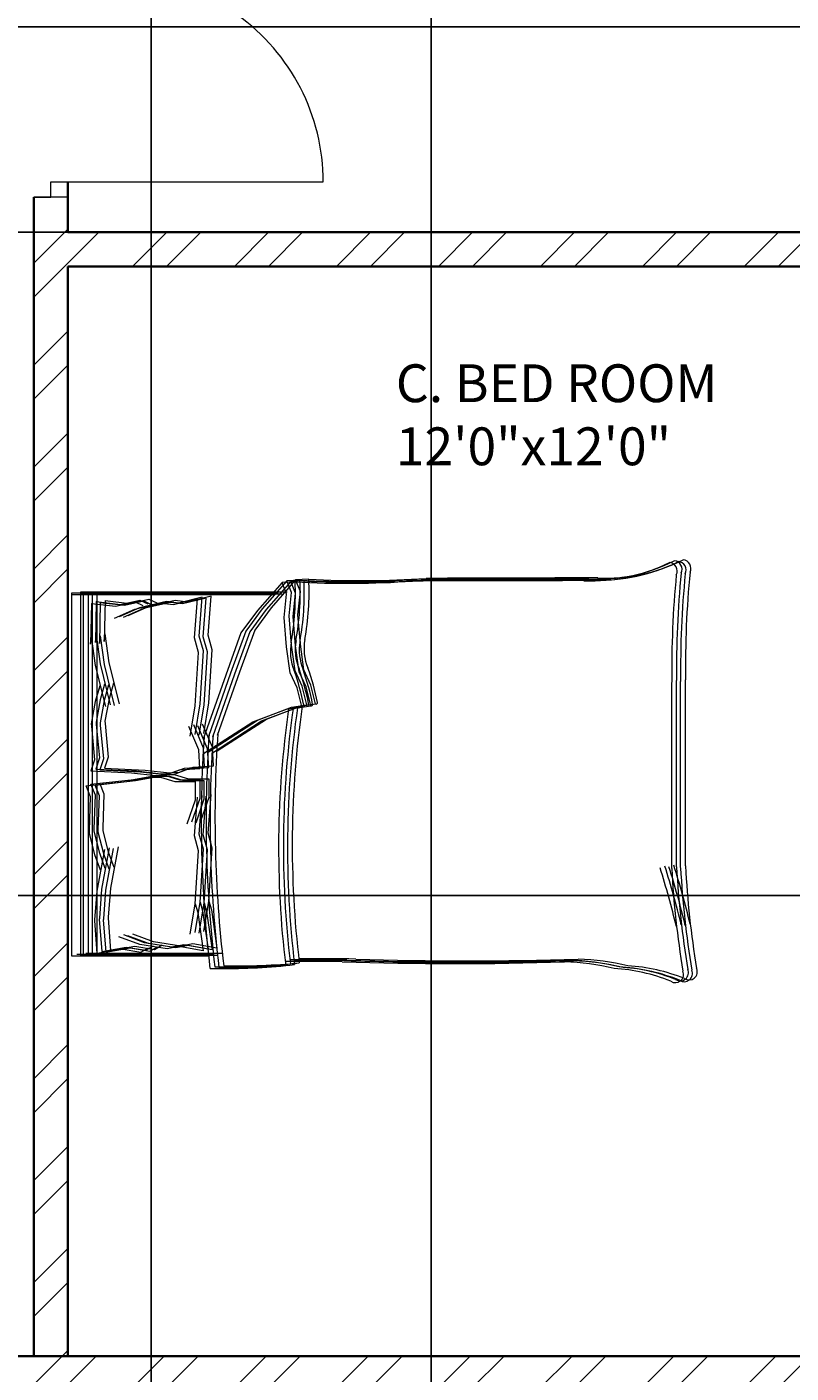
# Model space of a CAD drawing. Units: inches. Extents: x 1965 to 2673, y 1802 to 2669.
# Tile 14 of 16: x 2372 to 2473, y 2266 to 2444. Entities that reach past the tile are written whole.
import ezdxf

# ---------------------------------------------------------------- set-up
doc = ezdxf.new("R2010")
doc.units = ezdxf.units.IN
for name, color, linetype, lineweight in [('A-ANNO-DIMS', 2, 'Continuous', 18), ('A-AREA-IDEN', 7, 'Continuous', 18), ('A-DOOR', 11, 'Continuous', 18), ('A-FURN', 8, 'Continuous', 13), ('A-WALL', 7, 'Continuous', 35), ('A-WALL-PATT', 252, 'Continuous', 13)]:
    doc.layers.add(name, color=color, linetype=linetype, lineweight=lineweight)
doc.styles.get("Standard").update_dxf_attribs({"font": 'arial.ttf'})
doc.dimstyles.get("Standard").update_dxf_attribs({"dimtxt": 0.18, "dimasz": 0.18, "dimexe": 0.18, "dimexo": 0.0625, "dimgap": 0.09, "dimtad": 0, "dimtih": 1, "dimtoh": 1, "dimdec": 4, "dimzin": 0, "dimdsep": 46, "dimtxsty": 'Standard', "dimcen": 0.09, "dimadec": 0, "dimazin": 0, "dimtfac": 1, "dimtdec": 4, "dimtofl": 0, "dimtmove": 0, "dimatfit": 3, "dimfxl": 1, "dimtolj": 1, "dimtzin": 0, "dimarcsym": 0})

# ---------------------------------------------------------------- blocks, each defined once
blk = doc.blocks.new('BED-DOUBLE')
for p, q in [((3.47, 63.33), (3.47, 81.44)), ((3.47, 63.33), (3.47, 81.44)), ((3.47, 81.44), (51.49, 81.44)), ((3.7, 62.69), (3.7, 80.8)), ((3.7, 62.69), (3.7, 80.8)), ((51.26, 81.44), (51.26, 54.83)), ((51.26, 81.44), (51.26, 54.83)), ((51.49, 81.44), (51.49, 80.8)), ((51.49, 80.8), (51.49, 54.19)), ((51.49, 80.8), (51.49, 54.19)), ((3.47, 79.91), (51.26, 79.91)), ((3.47, 79.91), (51.26, 79.91)), ((3.7, 79.27), (51.49, 79.27)), ((3.7, 79.27), (51.49, 79.27)), ((3.89, 78.1), (8.17, 78.43)), ((3.89, 78.1), (8.17, 78.43)), ((8.17, 78.43), (8.28, 78.41)), ((8.17, 78.43), (8.28, 78.41)), ((8.28, 78.41), (12.1, 78.12)), ((8.28, 78.41), (12.1, 78.12)), ((14.85, 77.69), (16.87, 78.41)), ((14.85, 77.69), (16.87, 78.41)), ((16.87, 78.41), (19.76, 79.14)), ((16.87, 78.41), (19.76, 79.14)), ((17.1, 77.77), (19.99, 78.5)), ((17.1, 77.77), (19.99, 78.5)), ((19.76, 79.14), (20.09, 79.14)), ((19.76, 79.14), (20.09, 79.14)), ((19.99, 78.5), (20.31, 78.5)), ((19.99, 78.5), (20.31, 78.5)), ((20.09, 79.14), (24.53, 78.99)), ((20.09, 79.14), (24.53, 78.99)), ((20.31, 78.5), (24.76, 78.35)), ((20.31, 78.5), (24.76, 78.35)), ((24.53, 78.99), (25.98, 79.57)), ((24.53, 78.99), (25.98, 79.57)), ((24.76, 78.35), (26.21, 78.93)), ((24.76, 78.35), (26.21, 78.93)), ((25.98, 79.57), (26.56, 74.22)), ((25.98, 79.57), (26.56, 74.22)), ((26.21, 78.93), (26.78, 73.58)), ((26.21, 78.93), (26.78, 73.58)), ((27.97, 78.95), (27.73, 73.57)), ((27.97, 78.95), (27.73, 73.57)), ((28.2, 78.31), (27.96, 72.93)), ((28.2, 78.31), (27.96, 72.93)), ((29.45, 78.46), (27.97, 78.95)), ((29.45, 78.46), (27.97, 78.95)), ((29.68, 77.82), (28.2, 78.31)), ((29.68, 77.82), (28.2, 78.31)), ((33.88, 78.88), (29.45, 78.46)), ((33.88, 78.88), (29.45, 78.46)), ((34.2, 78.9), (33.88, 78.88)), ((34.2, 78.9), (33.88, 78.88)), ((37.13, 78.36), (34.2, 78.9)), ((37.13, 78.36), (34.2, 78.9)), ((41.91, 78.37), (36.49, 77.02)), ((41.91, 78.37), (36.49, 77.02)), ((39.2, 77.77), (37.13, 78.36)), ((39.19, 77.77), (37.13, 78.36)), ((45.71, 78.9), (41.91, 78.37)), ((45.71, 78.9), (41.91, 78.37)), ((50.11, 78.88), (44.7, 78.98)), ((44.7, 78.98), (45.71, 78.9)), ((50.11, 78.88), (44.7, 78.98)), ((44.7, 78.98), (45.71, 78.9)), ((50.34, 78.24), (44.93, 78.34)), ((44.93, 78.34), (45.94, 78.26)), ((50.34, 78.24), (44.93, 78.34)), ((44.93, 78.34), (45.94, 78.26)), ((50.11, 78.88), (49.73, 75.67)), ((50.11, 78.88), (49.73, 75.67)), ((3.89, 78.12), (4.47, 74.94)), ((3.89, 78.12), (4.47, 74.94)), ((4.12, 77.46), (8.4, 77.79)), ((4.12, 77.46), (8.4, 77.79)), ((4.12, 77.49), (4.7, 74.3)), ((4.12, 77.49), (4.7, 74.3)), ((8.4, 77.79), (8.51, 77.77)), ((8.4, 77.79), (8.51, 77.77)), ((8.51, 77.77), (12.33, 77.49)), ((8.51, 77.77), (12.33, 77.49)), ((12.1, 78.12), (17.6, 77.11)), ((12.1, 78.12), (17.6, 77.11)), ((12.33, 77.49), (17.82, 76.47)), ((12.33, 77.49), (17.82, 76.47)), ((15.08, 77.05), (17.1, 77.77)), ((15.08, 77.05), (17.1, 77.77)), ((34.11, 78.24), (29.68, 77.82)), ((34.11, 78.24), (29.68, 77.82)), ((34.43, 78.26), (34.11, 78.24)), ((34.43, 78.26), (34.11, 78.24)), ((37.36, 77.72), (34.43, 78.26)), ((37.36, 77.72), (34.43, 78.26)), ((42.14, 77.73), (36.72, 76.38)), ((42.14, 77.73), (36.72, 76.38)), ((39.42, 77.13), (37.36, 77.72)), ((39.42, 77.13), (37.36, 77.72)), ((45.94, 78.26), (42.14, 77.73)), ((45.94, 78.26), (42.14, 77.73)), ((50.34, 78.24), (49.96, 75.03)), ((50.34, 78.24), (49.96, 75.03)), ((4.47, 74.94), (4.03, 72.34)), ((4.47, 74.94), (4.03, 72.34)), ((5.05, 72.49), (6.06, 75.23)), ((5.05, 72.49), (6.06, 75.23)), ((49.3, 73.18), (48.12, 75.86)), ((49.3, 73.18), (48.12, 75.86)), ((49.53, 72.54), (48.35, 75.22)), ((49.53, 72.54), (48.35, 75.22)), ((49.73, 75.67), (50.32, 73.1)), ((49.73, 75.67), (50.32, 73.1)), ((49.96, 75.03), (50.55, 72.46)), ((49.96, 75.03), (50.55, 72.46)), ((4.7, 74.3), (4.26, 71.7)), ((4.7, 74.3), (4.26, 71.7)), ((5.27, 71.85), (6.29, 74.59)), ((5.27, 71.85), (6.29, 74.59)), ((26.56, 74.22), (27.13, 71.04)), ((26.56, 74.22), (27.13, 71.04)), ((26.78, 73.58), (27.36, 70.4)), ((26.78, 73.58), (27.36, 70.4)), ((27.73, 73.57), (27.35, 70.36)), ((27.73, 73.57), (27.35, 70.36)), ((27.96, 72.93), (27.58, 69.72)), ((27.96, 72.93), (27.58, 69.72)), ((50.11, 69.61), (49.3, 73.18)), ((50.11, 69.61), (49.3, 73.18)), ((50.32, 73.1), (49.81, 72.06)), ((50.32, 73.1), (49.81, 72.06)), ((4.03, 72.34), (4.61, 71.33)), ((4.03, 72.34), (4.61, 71.33)), ((4.26, 71.7), (4.84, 70.69)), ((4.26, 71.7), (4.84, 70.69)), ((4.47, 68.87), (5.05, 72.49)), ((4.47, 68.87), (5.05, 72.49)), ((4.7, 68.23), (5.27, 71.85)), ((4.7, 68.23), (5.27, 71.85)), ((50.34, 68.97), (49.53, 72.54)), ((50.34, 68.97), (49.53, 72.54)), ((50.55, 72.46), (50.04, 71.42)), ((50.55, 72.46), (50.04, 71.42)), ((27.13, 69.74), (26.56, 67.86)), ((27.13, 69.74), (26.56, 67.86)), ((27.13, 71.04), (27.13, 69.74)), ((27.13, 71.04), (27.13, 69.74)), ((27.35, 70.36), (27.43, 69.06)), ((27.35, 70.36), (27.43, 69.06)), ((27.36, 70.4), (27.36, 69.1)), ((27.36, 70.4), (27.36, 69.1)), ((27.58, 69.72), (27.66, 68.42)), ((27.58, 69.72), (27.66, 68.42)), ((49.92, 68.01), (50.11, 69.61)), ((49.92, 68.01), (50.11, 69.61)), ((4.76, 67.28), (4.47, 68.87)), ((4.76, 67.28), (4.47, 68.87)), ((4.99, 66.64), (4.7, 68.23)), ((4.99, 66.64), (4.7, 68.23)), ((26.56, 67.86), (26.56, 65.18)), ((26.56, 67.86), (26.56, 65.18)), ((27.36, 69.1), (26.78, 67.22)), ((27.36, 69.1), (26.78, 67.22)), ((27.43, 69.06), (28.13, 67.22)), ((27.43, 69.06), (28.13, 67.22)), ((27.66, 68.42), (28.35, 66.58)), ((27.66, 68.42), (28.35, 66.58)), ((50.69, 64.87), (49.92, 68.01)), ((50.69, 64.87), (49.92, 68.01)), ((50.15, 67.37), (50.34, 68.97)), ((50.15, 67.37), (50.34, 68.97)), ((4.18, 64.1), (4.76, 67.28)), ((4.18, 64.1), (4.76, 67.28)), ((4.41, 63.46), (4.99, 66.64)), ((4.41, 63.46), (4.99, 66.64)), ((24.1, 65.18), (20.95, 66.27)), ((24.1, 65.18), (20.95, 66.27)), ((26.78, 67.22), (26.78, 64.54)), ((26.78, 67.22), (26.78, 64.54)), ((28.13, 67.22), (28.29, 64.55)), ((28.13, 67.22), (28.29, 64.55)), ((28.35, 66.58), (28.52, 63.91)), ((28.35, 66.58), (28.52, 63.91)), ((30.75, 64.7), (33.82, 65.99)), ((30.75, 64.7), (33.82, 65.99)), ((50.92, 64.23), (50.15, 67.37)), ((50.92, 64.23), (50.15, 67.37)), ((9.28, 64.82), (4.18, 64.1)), ((9.28, 64.82), (4.18, 64.1)), ((9.5, 64.18), (4.41, 63.46)), ((9.5, 64.18), (4.41, 63.46)), ((6.38, 65.81), (10.41, 65.15)), ((6.38, 65.81), (10.41, 65.15)), ((6.6, 65.17), (10.64, 64.51)), ((6.61, 65.17), (10.64, 64.51)), ((10.41, 65.15), (9.28, 64.82)), ((10.41, 65.15), (9.28, 64.82)), ((10.64, 64.51), (9.5, 64.18)), ((10.64, 64.51), (9.5, 64.18)), ((10.41, 65.15), (17.42, 64.71)), ((10.41, 65.15), (17.42, 64.71)), ((10.64, 64.51), (17.65, 64.08)), ((10.64, 64.51), (17.65, 64.08)), ((17.42, 64.71), (19.38, 65.27)), ((17.42, 64.71), (19.38, 65.27)), ((17.65, 64.08), (19.61, 64.63)), ((17.65, 64.08), (19.61, 64.63)), ((19.38, 65.27), (24.51, 64.87)), ((19.38, 65.27), (24.51, 64.87)), ((19.61, 64.63), (24.74, 64.23)), ((19.61, 64.63), (24.74, 64.23)), ((24.33, 64.54), (21.18, 65.63)), ((24.33, 64.54), (21.18, 65.63)), ((26.56, 65.18), (24.1, 65.18)), ((26.56, 65.18), (24.1, 65.18)), ((26.78, 64.54), (24.33, 64.54)), ((26.78, 64.54), (24.33, 64.54)), ((28.29, 64.55), (30.75, 64.7)), ((28.29, 64.55), (30.75, 64.7)), ((28.52, 63.91), (30.97, 64.06)), ((28.52, 63.91), (30.97, 64.06)), ((30.25, 64.06), (34.44, 57.56)), ((30.25, 64.06), (34.44, 57.56)), ((30.97, 64.06), (34.04, 65.35)), ((30.97, 64.06), (34.04, 65.35)), ((40.64, 61.12), (32.3, 64.06)), ((40.64, 61.12), (32.3, 64.06)), ((32.56, 65.81), (36.59, 65.15)), ((32.56, 65.81), (36.59, 65.15)), ((32.79, 65.17), (36.82, 64.51)), ((32.79, 65.17), (36.82, 64.51)), ((36.59, 65.15), (43.6, 64.71)), ((36.59, 65.15), (43.6, 64.71)), ((36.82, 64.51), (43.83, 64.08)), ((36.82, 64.51), (43.83, 64.08)), ((43.6, 64.71), (45.56, 65.27)), ((43.6, 64.71), (45.56, 65.27)), ((43.83, 64.08), (45.79, 64.63)), ((43.83, 64.08), (45.79, 64.63)), ((45.56, 65.27), (50.69, 64.87)), ((45.56, 65.27), (50.69, 64.87)), ((45.79, 64.63), (50.92, 64.23)), ((45.79, 64.63), (50.92, 64.23)), ((30.48, 63.42), (34.67, 56.92)), ((30.48, 63.42), (34.67, 56.92)), ((40.87, 60.48), (32.53, 63.42)), ((40.87, 60.48), (32.53, 63.42)), ((46.21, 59.11), (40.64, 61.12)), ((46.21, 59.11), (40.64, 61.12)), ((46.44, 58.47), (40.87, 60.48)), ((46.44, 58.47), (40.87, 60.48)), ((49.16, 56.95), (46.21, 59.11)), ((49.16, 56.95), (46.21, 59.11)), ((34.44, 57.56), (36.15, 53.08)), ((34.44, 57.56), (36.15, 53.08)), ((34.67, 56.92), (36.38, 52.44)), ((34.67, 56.92), (36.38, 52.44)), ((49.39, 56.31), (46.44, 58.47)), ((49.39, 56.31), (46.44, 58.47)), ((52.86, 53.69), (49.16, 56.95)), ((52.86, 53.69), (49.16, 56.95)), ((53.09, 53.06), (49.39, 56.31)), ((53.09, 53.06), (49.39, 56.31)), ((44.36, 53.08), (48.23, 53.39)), ((44.36, 53.08), (48.23, 53.39)), ((48.23, 53.39), (51.33, 53.08)), ((48.23, 53.39), (51.33, 53.08)), ((51.33, 53.08), (52.86, 53.69)), ((51.33, 53.08), (52.86, 53.69)), ((52.94, 51.95), (52.86, 53.69, 3.87)), ((52.94, 51.95), (52.86, 53.69, 3.87)), ((36.15, 53.08), (36.46, 51.06)), ((36.15, 53.08), (36.46, 51.06)), ((36.38, 52.44), (36.69, 50.42)), ((36.38, 52.44), (36.69, 50.42)), ((36.46, 51.06), (38.94, 51.68)), ((36.46, 51.06), (38.94, 51.68)), ((38.94, 51.68), (40.95, 52.61)), ((38.94, 51.68), (40.95, 52.61)), ((39.16, 51.04), (41.18, 51.97)), ((39.16, 51.04), (41.18, 51.97)), ((40.95, 52.61), (44.36, 53.08)), ((40.95, 52.61), (44.36, 53.08)), ((41.18, 51.97), (44.58, 52.44)), ((41.18, 51.97), (44.58, 52.44)), ((44.58, 52.44), (48.46, 52.75)), ((44.58, 52.44), (48.46, 52.75)), ((48.46, 52.75), (51.55, 52.44)), ((48.46, 52.75), (51.55, 52.44)), ((51.55, 52.44), (53.09, 53.06)), ((51.55, 52.44), (53.09, 53.06)), ((53.17, 51.31), (53.09, 53.06, 3.87)), ((53.17, 51.31), (53.09, 53.06, 3.87)), ((36.69, 50.42), (39.16, 51.04)), ((36.69, 50.42), (39.16, 51.04)), ((15.06, 2.2), (39.67, 2.2)), ((15.06, 2.2), (39.67, 2.2)), ((15.29, 1.56), (39.9, 1.56)), ((15.29, 1.56), (39.9, 1.56))]:
    blk.add_line(p, q)
for centre, radius, start, end in [((21.35, -100.61), 164.97, 86.0865, 96.7821), ((21.35, -100.61), 164.97, 86.0865, 96.7821), ((85.16, 61.34), 83.31, 178.7218, 185.604), ((85.16, 61.34), 83.31, 178.7218, 185.604), ((85.39, 60.71), 83.31, 178.7218, 185.604), ((85.38, 60.71), 83.31, 178.7218, 185.604), ((21.58, -101.25), 164.97, 86.0865, 96.7821), ((21.58, -101.25), 164.97, 86.0865, 96.7821), ((17.75, -74.88), 129.02, 81.7845, 96.9006), ((17.75, -74.88), 129.02, 81.7845, 96.9006), ((17.98, -75.51), 129.02, 81.7845, 96.9006), ((17.98, -75.51), 129.02, 81.7845, 96.9006), ((-167.31, 50.27), 170.11, 358.4762, 1.0082), ((-167.31, 50.27), 170.11, 358.4762, 1.0082), ((-167.08, 49.63), 170.11, 358.4762, 1.0082), ((-167.08, 49.63), 170.11, 358.4762, 1.0082), ((31.15, 79.96), 29.65, 280.6617, 289.8806), ((31.15, 79.96), 29.65, 280.6617, 289.8806), ((43.74, 46.37), 6.22, 78.6608, 113.7384), ((43.74, 46.37), 6.22, 78.6608, 113.7384), ((43.97, 45.74), 6.22, 78.6608, 113.7384), ((43.97, 45.74), 6.22, 78.6608, 113.7384), ((51.32, 88.1), 36.18, 259.8763, 272.5657), ((51.32, 88.1), 36.18, 259.8763, 272.5657), ((51.55, 87.46), 36.18, 259.8763, 272.5657), ((51.55, 87.46), 36.18, 259.8763, 272.5657), ((182.26, 45.13), 129.5, 176.9791, 183.8365), ((182.26, 45.13), 129.5, 176.9791, 183.8365), ((36.63, 51), 0.185, 160.2464, 271.1377), ((36.63, 51), 0.185, 160.2464, 271.1377), ((36.86, 50.36), 0.185, 160.2464, 271.1377), ((36.86, 50.36), 0.185, 160.2464, 271.1377), ((31.38, 79.32), 29.65, 280.6617, 289.8806), ((31.38, 79.32), 29.65, 280.6617, 289.8806), ((182.49, 44.49), 129.5, 176.9791, 183.8365), ((182.49, 44.49), 129.5, 176.9791, 183.8365), ((484.82, 30.83), 482.31, 178.2277, 181.7185), ((484.82, 30.83), 482.31, 178.2277, 181.7185), ((485.05, 30.19), 482.31, 178.2277, 181.7185), ((485.05, 30.19), 482.31, 178.2277, 181.7185), ((-4508.75, 13.62), 4561.86, 0.00217, 0.28689), ((-4508.75, 13.62), 4561.86, 0.00217, 0.28689), ((-4508.52, 12.98), 4561.86, 0.00217, 0.28689), ((-4508.52, 12.98), 4561.86, 0.00217, 0.28689), ((-26.9, 16.93), 29.63, 346.0648, 358.9113), ((-26.9, 16.93), 29.63, 346.0648, 358.9113), ((-26.68, 16.29), 29.63, 346.0648, 358.9113), ((-26.68, 16.29), 29.63, 346.0648, 358.9113), ((76.15, 12.77), 23.07, 177.4714, 206.4681), ((76.15, 12.77), 23.07, 177.4714, 206.4681), ((76.38, 12.14), 23.07, 177.4714, 206.4681), ((76.38, 12.14), 23.07, 177.4714, 206.4681), ((-21.66, 11.17), 23.56, 337.9751, 356.652), ((-21.66, 11.17), 23.56, 337.9751, 356.652), ((-21.44, 10.53), 23.56, 337.9751, 356.652), ((-21.44, 10.53), 23.56, 337.9751, 356.652), ((-17.23, 105.15), 106.46, 283.3832, 287.7053), ((-17.23, 105.15), 106.46, 283.3832, 287.7053), ((1.08, 1.72), 1.09, 146.1736, 293.4781), ((1.08, 1.72), 1.09, 146.1736, 293.4781), ((21.42, -119.4), 121.76, 92.9958, 99.4091), ((21.42, -119.4), 121.76, 92.9958, 99.4091), ((-17, 104.51), 106.46, 283.3832, 287.7053), ((-17, 104.51), 106.46, 283.3832, 287.7053), ((41.15, -130.84), 133.04, 84.4998, 90.6351), ((41.15, -130.84), 133.04, 84.4998, 90.6351), ((54.4, 2.57), 1.1, 242.6588, 356.02), ((54.4, 2.57), 1.1, 242.6588, 356.02), ((54.63, 1.93), 1.1, 242.6588, 356.02), ((54.63, 1.93), 1.1, 242.6588, 356.02), ((1.31, 1.08), 1.09, 146.1736, 293.4781), ((1.31, 1.08), 1.09, 146.1736, 293.4781), ((21.65, -120.04), 121.76, 92.9958, 99.4091), ((21.65, -120.04), 121.76, 92.9958, 99.4091), ((41.38, -131.48), 133.04, 84.4998, 90.6351), ((41.37, -131.48), 133.04, 84.4998, 90.6351)]:
    blk.add_arc(centre, radius, start, end)
blk = doc.blocks.new('*D48')
at = {"layer": 'A-ANNO-DIMS', "color": 0, "lineweight": -2, "transparency": 16777216}
for p, q in [((2573.53, 2329.47), (2012.19, 2329.47)), ((2012.37, 2329.29), (2012.37, 2299.21)), ((2012.37, 2268.77), (2012.37, 2298.85)), ((2573.53, 2268.59), (2012.19, 2268.59))]:
    blk.add_line(p, q, dxfattribs=at)
at = {"layer": 'A-ANNO-DIMS', "color": 0, "transparency": 16777216}
for points in [[(2012.34, 2329.29), (2012.4, 2329.29), (2012.37, 2329.47)], [(2012.34, 2268.77), (2012.4, 2268.77), (2012.37, 2268.59)]]:
    blk.add_solid(points, dxfattribs=at)
at = {"layer": 'Defpoints', "color": 0, "transparency": 16777216}
for p in [(2012.37, 2329.47), (2573.59, 2329.47), (2573.59, 2268.59)]:
    blk.add_point(p, dxfattribs=at)
at = {"layer": 'A-ANNO-DIMS', "color": 0, "transparency": 16777216, "insert": (2012.37, 2299.03), "char_height": 0.18, "attachment_point": 5}
blk.add_mtext('\\A1;60.87', dxfattribs=at)
blk = doc.blocks.new('*D49')
at = {"layer": 'A-ANNO-DIMS', "color": 0, "lineweight": -2, "transparency": 16777216}
for p, q in [((2573.53, 2444.23), (2012.19, 2444.23)), ((2012.37, 2444.05), (2012.37, 2430.84)), ((2012.37, 2417.27), (2012.37, 2430.48)), ((2573.53, 2417.09), (2012.19, 2417.09))]:
    blk.add_line(p, q, dxfattribs=at)
at = {"layer": 'A-ANNO-DIMS', "color": 0, "transparency": 16777216}
for points in [[(2012.34, 2444.05), (2012.4, 2444.05), (2012.37, 2444.23)], [(2012.34, 2417.27), (2012.4, 2417.27), (2012.37, 2417.09)]]:
    blk.add_solid(points, dxfattribs=at)
at = {"layer": 'Defpoints', "color": 0, "transparency": 16777216}
for p in [(2012.37, 2444.23), (2573.59, 2444.23), (2573.59, 2417.09)]:
    blk.add_point(p, dxfattribs=at)
at = {"layer": 'A-ANNO-DIMS', "color": 0, "transparency": 16777216, "insert": (2012.37, 2430.66), "char_height": 0.18, "attachment_point": 5}
blk.add_mtext('\\A1;27.137', dxfattribs=at)
blk = doc.blocks.new('*D50')
at = {"layer": 'A-ANNO-DIMS', "color": 0, "lineweight": -2, "transparency": 16777216}
for p, q in [((2388.09, 2116.15), (2388.09, 2600.5)), ((2388.27, 2600.32), (2406.37, 2600.32)), ((2424.91, 2600.32), (2406.81, 2600.32)), ((2425.09, 2116.15), (2425.09, 2600.5))]:
    blk.add_line(p, q, dxfattribs=at)
at = {"layer": 'A-ANNO-DIMS', "color": 0, "transparency": 16777216}
for points in [[(2388.27, 2600.35), (2388.27, 2600.29), (2388.09, 2600.32)], [(2424.91, 2600.35), (2424.91, 2600.29), (2425.09, 2600.32)]]:
    blk.add_solid(points, dxfattribs=at)
at = {"layer": 'Defpoints', "color": 0, "transparency": 16777216}
for p in [(2425.09, 2600.32), (2388.09, 2116.09), (2425.09, 2116.09)]:
    blk.add_point(p, dxfattribs=at)
at = {"layer": 'A-ANNO-DIMS', "color": 0, "transparency": 16777216, "insert": (2406.59, 2600.32), "char_height": 0.18, "attachment_point": 5}
blk.add_mtext('\\A1;37', dxfattribs=at)

msp = doc.modelspace()

# ---------------------------------------------------------------- hatches: boundary and pattern name
at = {"layer": 'A-WALL-PATT'}
h = msp.add_hatch(dxfattribs=at)
h.set_pattern_fill('ANSI32', color=256)
h.paths.add_polyline_path([(2051.5927, 2561.0914), (2076.7559, 2561.0914), (2076.7559, 2563.3414), (2076.7559, 2565.5914), (2047.0927, 2565.5914), (2047.0927, 2518.3824), (2051.5927, 2518.3824)])
h.paths.add_polyline_path([(2051.5927, 2458.3824), (2049.3427, 2458.3824), (2047.0927, 2458.3824), (2047.0927, 2412.5914), (2248.0927, 2412.5914), (2248.0927, 2268.5914), (2252.5927, 2268.5914), (2252.5927, 2412.5914), (2252.5927, 2421.0404), (2250.3427, 2421.0404), (2248.0927, 2421.0404), (2248.0927, 2417.0914), (2051.5927, 2417.0914)])
h.paths.add_polyline_path([(2211.4933, 2268.5914), (2104.0927, 2268.5914), (2104.0927, 2272.4654), (2101.8427, 2272.4654), (2099.5927, 2272.4654), (2099.5927, 2268.5914), (2051.5927, 2268.5914), (2051.5927, 2264.0914), (2147.5927, 2264.0914), (2147.5927, 2259.8893), (2152.0927, 2259.8893), (2152.0927, 2264.0914), (2211.4933, 2264.0914), (2211.4933, 2266.3414)])
h.paths.add_polyline_path([(2104.0927, 2376.0914), (2099.5927, 2376.0914), (2047.0927, 2376.0914), (2047.0927, 2333.0682), (2051.5927, 2333.0682), (2051.5927, 2371.5914), (2099.5927, 2371.5914), (2099.5927, 2293.6123), (2104.0927, 2293.6123)], flags=17)
h.paths.add_polyline_path([(2051.5927, 2309.0682), (2047.0927, 2309.0682), (2047.0927, 2233.5821), (2051.5927, 2233.5821)])
h.paths.add_polyline_path([(2104.0927, 2412.5914), (2099.5927, 2412.5914), (2099.5927, 2376.0914), (2104.0927, 2376.0914)], flags=17)
h.paths.add_polyline_path([(2290.1254, 2268.5914), (2242.4924, 2268.5914), (2242.4924, 2264.0914), (2290.1254, 2264.0914), (2290.1254, 2266.3414)])
h.paths.add_polyline_path([(2284.653, 2264.0914), (2280.153, 2264.0914), (2280.153, 2161.6826), (2284.653, 2161.6826)])
h.paths.add_polyline_path([(2578.0927, 2329.4656), (2573.5927, 2329.4656), (2573.5927, 2268.5914), (2525.5927, 2268.5914), (2525.5927, 2271.9222), (2523.3427, 2271.9222), (2521.0927, 2271.9222), (2521.0927, 2268.5914), (2324.2835, 2268.5914), (2324.2835, 2264.0914), (2329.0927, 2264.0914), (2329.0927, 2259.4977), (2333.5927, 2259.4977), (2333.5927, 2264.0914), (2473.0927, 2264.0914), (2473.0927, 2259.9371), (2477.5927, 2259.9371), (2477.5927, 2264.0914), (2573.5927, 2264.0914), (2573.5927, 2235.5751), (2578.0927, 2235.5751)])
h.paths.add_polyline_path([(2377.0927, 2412.5914), (2578.0927, 2412.5914), (2578.0927, 2444.2286), (2575.8427, 2444.2286), (2573.5927, 2444.2286), (2573.5927, 2417.0914), (2429.5927, 2417.0914), (2377.0927, 2417.0914), (2377.0927, 2421.7443), (2372.5927, 2421.7443), (2372.5927, 2268.5914), (2377.0927, 2268.5914)])
h.paths.add_polyline_path([(2525.5927, 2371.5914), (2573.5927, 2371.5914), (2573.5927, 2353.4656), (2578.0927, 2353.4656), (2578.0927, 2376.0914), (2525.5927, 2376.0914), (2521.0927, 2376.0914), (2521.0927, 2290.6472), (2525.5927, 2290.6472)], flags=17)
h.paths.add_polyline_path([(2477.5927, 2236.4106), (2475.3427, 2236.4106), (2473.0927, 2236.4106), (2473.0927, 2084.5914), (2465.3309, 2084.5914), (2465.3309, 2080.0914), (2481.6764, 2080.0914), (2481.6764, 2082.3414), (2481.6764, 2084.5914), (2477.5927, 2084.5914), (2477.5927, 2151.5914), (2573.5927, 2151.5914), (2573.5927, 2130.2907), (2578.0927, 2130.2907), (2578.0927, 2199.5751), (2575.8427, 2199.5751), (2573.5927, 2199.5751), (2573.5927, 2156.0914), (2477.5927, 2156.0914)])
h.paths.add_polyline_path([(2573.5927, 2084.5914), (2505.5513, 2084.5914), (2505.5513, 2080.0914), (2573.5927, 2080.0914)], flags=17)
h.paths.add_polyline_path([(2578.0927, 2106.2907), (2575.8427, 2106.2907), (2573.5927, 2106.2907), (2573.5927, 2050.8986), (2578.0927, 2050.8986)])
h.paths.add_polyline_path([(2578.0927, 1990.8986), (2575.8427, 1990.8986), (2573.5927, 1990.8986), (2573.5927, 1936.0914), (2522.132, 1936.0914), (2522.132, 1931.5914), (2578.0927, 1931.5914)])
h.paths.add_polyline_path([(2462.132, 1936.0914), (2429.5927, 1936.0914), (2429.5927, 2080.0914), (2432.623, 2080.0914), (2432.623, 2082.3414), (2432.623, 2084.5914), (2429.5927, 2084.5914), (2429.5927, 2120.5914), (2333.5927, 2120.5914), (2333.5927, 2229.3125), (2331.3427, 2229.3125), (2329.0927, 2229.3125), (2329.0927, 2116.0914), (2425.0927, 2116.0914), (2425.0927, 1936.0914), (2346.4058, 1936.0914), (2346.4058, 1931.5914), (2462.132, 1931.5914), (2462.132, 1933.8414)])
h.paths.add_polyline_path([(2211.767, 1933.8414), (2211.767, 1936.0914), (2200.0927, 1936.0914), (2200.0927, 2080.0914), (2200.0927, 2116.0914), (2284.653, 2116.0914), (2284.653, 2130.591), (2282.403, 2130.591), (2280.153, 2130.591), (2280.153, 2120.5914), (2200.0927, 2120.5914), (2195.5927, 2120.5914), (2195.5927, 2080.0914), (2195.5927, 1936.0914), (2139.0533, 1936.0914), (2139.0533, 1931.5914), (2211.767, 1931.5914)])
h.paths.add_polyline_path([(2282.2502, 1933.8414), (2282.2502, 1936.0914), (2259.767, 1936.0914), (2259.767, 1931.5914), (2282.2502, 1931.5914)], flags=17)
h.paths.add_polyline_path([(2051.5927, 1987.096), (2049.3427, 1987.096), (2047.0927, 1987.096), (2047.0927, 1931.5914), (2079.0533, 1931.5914), (2079.0533, 1933.8414), (2079.0533, 1936.0914), (2051.5927, 1936.0914)])
h.paths.add_polyline_path([(2051.5927, 2197.5821), (2049.3427, 2197.5821), (2047.0927, 2197.5821), (2047.0927, 2141.952), (2051.5927, 2141.952), (2051.5927, 2151.5914), (2147.5927, 2151.5914), (2147.5927, 2084.5914), (2144.3652, 2084.5914), (2144.3652, 2080.0914), (2155.9662, 2080.0914), (2155.9662, 2082.3414), (2155.9662, 2084.5914), (2152.0927, 2084.5914), (2152.0927, 2239.4921), (2149.8427, 2239.4921), (2147.5927, 2239.4921), (2147.5927, 2156.0914), (2051.5927, 2156.0914)])
h.paths.add_polyline_path([(2051.5927, 2080.0914), (2123.8575, 2080.0914), (2123.8575, 2082.3414), (2123.8575, 2084.5914), (2051.5927, 2084.5914), (2051.5927, 2117.952), (2047.0927, 2117.952), (2047.0927, 2047.096), (2051.5927, 2047.096)])
h = msp.add_hatch(dxfattribs=at)
h.set_pattern_fill('ANSI32', color=256)
h.paths.add_polyline_path([(2210.2316, 2563.3414), (2210.2316, 2565.5914), (2136.7559, 2565.5914), (2136.7559, 2561.0914), (2195.5927, 2561.0914), (2195.5927, 2485.8604), (2200.0927, 2485.8604), (2200.0927, 2561.0914), (2210.2316, 2561.0914)])
h.paths.add_polyline_path([(2285.9734, 2565.5914), (2234.2316, 2565.5914), (2234.2316, 2561.0914), (2248.0927, 2561.0914), (2248.0927, 2462.0914), (2200.0927, 2462.0914), (2200.0927, 2465.2357), (2197.8427, 2465.2357), (2195.5927, 2465.2357), (2195.5927, 2457.5914), (2248.0927, 2457.5914), (2248.0927, 2452.628), (2252.5927, 2452.628), (2252.5927, 2457.5914), (2257.5156, 2457.5914), (2257.5156, 2459.8414), (2257.5156, 2462.0914), (2252.5927, 2462.0914), (2252.5927, 2561.0914), (2285.9734, 2561.0914)])
h.paths.add_polyline_path([(2213.1374, 1872.8885), (2461.061, 1872.8885), (2461.061, 1909.9813), (2213.1374, 1909.9813)], flags=9)
h.paths.add_polyline_path([(2328.4056, 1942.3944), (2340.6089, 1942.3944), (2340.6089, 1952.6979), (2328.4056, 1952.6979)], flags=9)
h.paths.add_polyline_path([(2353.5759, 2030.9808), (2376.6455, 2030.9808), (2376.6455, 2041.2844), (2353.5759, 2041.2844)], flags=9)
h.paths.add_polyline_path([(2289.989, 2074.1041), (2326.916, 2074.1041), (2326.916, 2092.7615), (2289.989, 2092.7615)], flags=9)
h.paths.add_polyline_path([(2497.9, 2052.8638), (2548.3741, 2052.8638), (2548.3741, 2071.5212), (2497.9, 2071.5212)], flags=9)
h.paths.add_polyline_path([(2486.59, 2116.4883), (2515.7475, 2116.4883), (2515.7475, 2135.1456), (2486.59, 2135.1456)], flags=9)
h.paths.add_polyline_path([(2497.3007, 2181.2877), (2530.459, 2181.2877), (2530.459, 2199.945), (2497.3007, 2199.945)], flags=9)
h.paths.add_polyline_path([(2288.237, 2190.3228), (2324.1238, 2190.3228), (2324.1238, 2208.9802), (2288.237, 2208.9802)], flags=9)
h.paths.add_polyline_path([(2350.806, 2127.8307), (2387.733, 2127.8307), (2387.733, 2146.488), (2350.806, 2146.488)], flags=9)
h.paths.add_polyline_path([(2530.3237, 2315.2679), (2559.5563, 2315.2679), (2559.5563, 2333.9252), (2530.3237, 2333.9252)], flags=9)
h.paths.add_polyline_path([(2418.419, 2383.4707), (2468.2894, 2383.4707), (2468.2894, 2402.1281), (2418.419, 2402.1281)], flags=9)
h.paths.add_polyline_path([(2327.4503, 2399.0281), (2364.3773, 2399.0281), (2364.3773, 2417.6854), (2327.4503, 2417.6854)], flags=9)
h.paths.add_polyline_path([(2147.9722, 2271.4601), (2197.8426, 2271.4601), (2197.8426, 2290.1174), (2147.9722, 2290.1174)], flags=9)
h.paths.add_polyline_path([(2474.3875, 2421.594), (2524.8616, 2421.594), (2524.8616, 2440.2514), (2474.3875, 2440.2514)], flags=9)
h.paths.add_polyline_path([(2063.9863, 2052.9059), (2114.4604, 2052.9059), (2114.4604, 2071.5632), (2063.9863, 2071.5632)], flags=9)
h.paths.add_polyline_path([(2200.3335, 2133.7067), (2237.2605, 2133.7067), (2237.2605, 2152.364), (2200.3335, 2152.364)], flags=9)
h.paths.add_polyline_path([(2080.5973, 2184.636), (2113.8681, 2184.636), (2113.8681, 2203.2933), (2080.5973, 2203.2933)], flags=9)
h.paths.add_polyline_path([(2102.4918, 2116.4497), (2131.6494, 2116.4497), (2131.6494, 2135.107), (2102.4918, 2135.107)], flags=9)
h.paths.add_polyline_path([(2056.2753, 2308.5576), (2085.5079, 2308.5576), (2085.5079, 2327.2149), (2056.2753, 2327.2149)], flags=9)
h.paths.add_polyline_path([(2385.619, 2500.9729), (2414.8516, 2500.9729), (2414.8516, 2519.6303), (2385.619, 2519.6303)], flags=9)
h.paths.add_polyline_path([(2286.6643, 2508.6826), (2320.0715, 2508.6826), (2320.0715, 2527.34), (2286.6643, 2527.34)], flags=9)
h.paths.add_polyline_path([(2206.5604, 2500.7243), (2235.793, 2500.7243), (2235.793, 2519.3817), (2206.5604, 2519.3817)], flags=25)
h.paths.add_polyline_path([(2062.6644, 2424.4027), (2112.5348, 2424.4027), (2112.5348, 2443.0601), (2062.6644, 2443.0601)], flags=9)
h = msp.add_hatch(dxfattribs=at)
h.set_pattern_fill('ANSI32', color=256)
h.paths.add_polyline_path([(2429.5927, 2468.6101), (2427.3427, 2468.6101), (2425.0927, 2468.6101), (2425.0927, 2462.0914), (2377.0927, 2462.0914), (2377.0927, 2561.0914), (2390.4173, 2561.0914), (2390.4173, 2565.5914), (2321.9734, 2565.5914), (2321.9734, 2561.0914), (2372.5927, 2561.0914), (2372.5927, 2462.0914), (2281.6605, 2462.0914), (2281.6605, 2457.5914), (2372.5927, 2457.5914), (2372.5927, 2451.3316), (2377.0927, 2451.3316), (2377.0927, 2457.5914), (2429.5927, 2457.5914)])
h.paths.add_polyline_path([(2480.8929, 2565.5914), (2414.4173, 2565.5914), (2414.4173, 2561.0914), (2425.0927, 2561.0914), (2425.0927, 2489.9153), (2429.5927, 2489.9153), (2429.5927, 2561.0914), (2480.8929, 2561.0914), (2480.8929, 2563.3414)])
h.paths.add_polyline_path([(2213.1374, 1872.8885), (2461.061, 1872.8885), (2461.061, 1909.9813), (2213.1374, 1909.9813)], flags=9)
h.paths.add_polyline_path([(2328.4056, 1942.3944), (2340.6089, 1942.3944), (2340.6089, 1952.6979), (2328.4056, 1952.6979)], flags=9)
h.paths.add_polyline_path([(2353.5759, 2030.9808), (2376.6455, 2030.9808), (2376.6455, 2041.2844), (2353.5759, 2041.2844)], flags=9)
h.paths.add_polyline_path([(2289.989, 2074.1041), (2326.916, 2074.1041), (2326.916, 2092.7615), (2289.989, 2092.7615)], flags=9)
h.paths.add_polyline_path([(2497.9, 2052.8638), (2548.3741, 2052.8638), (2548.3741, 2071.5212), (2497.9, 2071.5212)], flags=9)
h.paths.add_polyline_path([(2486.59, 2116.4883), (2515.7475, 2116.4883), (2515.7475, 2135.1456), (2486.59, 2135.1456)], flags=9)
h.paths.add_polyline_path([(2497.3007, 2181.2877), (2530.459, 2181.2877), (2530.459, 2199.945), (2497.3007, 2199.945)], flags=9)
h.paths.add_polyline_path([(2288.237, 2190.3228), (2324.1238, 2190.3228), (2324.1238, 2208.9802), (2288.237, 2208.9802)], flags=9)
h.paths.add_polyline_path([(2350.806, 2127.8307), (2387.733, 2127.8307), (2387.733, 2146.488), (2350.806, 2146.488)], flags=9)
h.paths.add_polyline_path([(2530.3237, 2315.2679), (2559.5563, 2315.2679), (2559.5563, 2333.9252), (2530.3237, 2333.9252)], flags=9)
h.paths.add_polyline_path([(2418.419, 2383.4707), (2468.2894, 2383.4707), (2468.2894, 2402.1281), (2418.419, 2402.1281)], flags=9)
h.paths.add_polyline_path([(2327.4503, 2399.0281), (2364.3773, 2399.0281), (2364.3773, 2417.6854), (2327.4503, 2417.6854)], flags=9)
h.paths.add_polyline_path([(2147.9722, 2271.4601), (2197.8426, 2271.4601), (2197.8426, 2290.1174), (2147.9722, 2290.1174)], flags=9)
h.paths.add_polyline_path([(2474.3875, 2421.594), (2524.8616, 2421.594), (2524.8616, 2440.2514), (2474.3875, 2440.2514)], flags=9)
h.paths.add_polyline_path([(2063.9863, 2052.9059), (2114.4604, 2052.9059), (2114.4604, 2071.5632), (2063.9863, 2071.5632)], flags=9)
h.paths.add_polyline_path([(2200.3335, 2133.7067), (2237.2605, 2133.7067), (2237.2605, 2152.364), (2200.3335, 2152.364)], flags=9)
h.paths.add_polyline_path([(2080.5973, 2184.636), (2113.8681, 2184.636), (2113.8681, 2203.2933), (2080.5973, 2203.2933)], flags=9)
h.paths.add_polyline_path([(2102.4918, 2116.4497), (2131.6494, 2116.4497), (2131.6494, 2135.107), (2102.4918, 2135.107)], flags=9)
h.paths.add_polyline_path([(2056.2753, 2308.5576), (2085.5079, 2308.5576), (2085.5079, 2327.2149), (2056.2753, 2327.2149)], flags=9)
h.paths.add_polyline_path([(2385.619, 2500.9729), (2414.8516, 2500.9729), (2414.8516, 2519.6303), (2385.619, 2519.6303)], flags=25)
h.paths.add_polyline_path([(2286.6643, 2508.6826), (2320.0715, 2508.6826), (2320.0715, 2527.34), (2286.6643, 2527.34)], flags=25)
h.paths.add_polyline_path([(2206.5604, 2500.7243), (2235.793, 2500.7243), (2235.793, 2519.3817), (2206.5604, 2519.3817)], flags=9)
h.paths.add_polyline_path([(2062.6644, 2424.4027), (2112.5348, 2424.4027), (2112.5348, 2443.0601), (2062.6644, 2443.0601)], flags=9)

# ---------------------------------------------------------------- linework, layer by layer
at = {"layer": 'A-DOOR'}
for p, q in [((2374.8427, 2421.7443), (2374.8427, 2423.7443)), ((2374.8427, 2423.7443), (2410.8427, 2423.7443)), ((2377.0927, 2421.7443), (2372.5927, 2421.7443)), ((2372.5927, 2421.7443), (2374.8427, 2421.7443))]:
    msp.add_line(p, q, dxfattribs=at)
msp.add_arc((2383.7495, 2423.7443), 27.0932, 360, 109.192689, dxfattribs=at)
at = {"layer": 'A-WALL'}
for p, q in [((2377.0927, 2423.7443), (2377.0927, 2417.0914)), ((2372.5927, 2421.7443), (2372.5927, 2268.5914)), ((2377.0927, 2417.0914), (2573.5927, 2417.0914)), ((2429.5927, 2417.0914), (2573.5927, 2417.0914)), ((2372.5927, 2412.5914), (2372.5927, 2268.5914)), ((2377.0927, 2412.5914), (2377.0927, 2268.5914)), ((2377.0927, 2412.5914), (2578.0927, 2412.5914)), ((2322.5984, 2268.5914), (2521.0927, 2268.5914))]:
    msp.add_line(p, q, dxfattribs=at)

# ---------------------------------------------------------------- block references
at = {"layer": 'A-FURN'}
for p, rotation in [((2459.0774, 2317.945), 89.99999983318573), ((2460.2503, 2318.0717), 89.99999983318561)]:
    msp.add_blockref('BED-DOUBLE', p, dxfattribs=dict(at, rotation=rotation))

# ---------------------------------------------------------------- texts
at = {"layer": 'A-AREA-IDEN', "insert": (2420.4296, 2399.6434), "char_height": 5, "attachment_point": 1}
msp.add_mtext_dynamic_manual_height_columns('C. BED ROOM\\P12\'0"x12\'0"', width=339.509662, gutter_width=12.5, heights=[0], dxfattribs=at)

# ---------------------------------------------------------------- dimensions: what is measured, and where the dimension line sits
at = {"layer": 'A-ANNO-DIMS'}
dim = msp.add_linear_dim(base=(2425.0927, 2600.3164), p1=(2388.0925, 2116.0914), p2=(2425.0927, 2116.0914), dimstyle='Standard', override={"dimdec": 0, "dimlfac": 1, "dimrnd": 0, "dimzin": 0, "dimdsep": 46, "dimlunit": 2}, dxfattribs=at)
dim.commit()
dim.dimension.update_dxf_attribs({"geometry": '*D50', "text_midpoint": (2406.5926, 2600.3164)})
for base, p1, p2, override, picture, middle in [((2012.3677, 2444.2286), (2573.5927, 2417.0914), (2573.5927, 2444.2286), {"dimdec": 3, "dimlfac": 1, "dimrnd": 0, "dimzin": 0, "dimdsep": 46, "dimlunit": 2}, '*D49', (2012.3677, 2430.66)), ((2012.3677, 2329.4656), (2573.5927, 2268.5914), (2573.5927, 2329.4656), {"dimdec": 2, "dimlfac": 1, "dimrnd": 0, "dimzin": 0, "dimdsep": 46, "dimlunit": 2}, '*D48', (2012.3677, 2299.0285))]:
    dim = msp.add_linear_dim(base=base, p1=p1, p2=p2, angle=90, dimstyle='Standard', override=override, dxfattribs=at)
    dim.commit()
    dim.dimension.update_dxf_attribs({"geometry": picture, "text_midpoint": middle})

doc.saveas('drawing.dxf')
